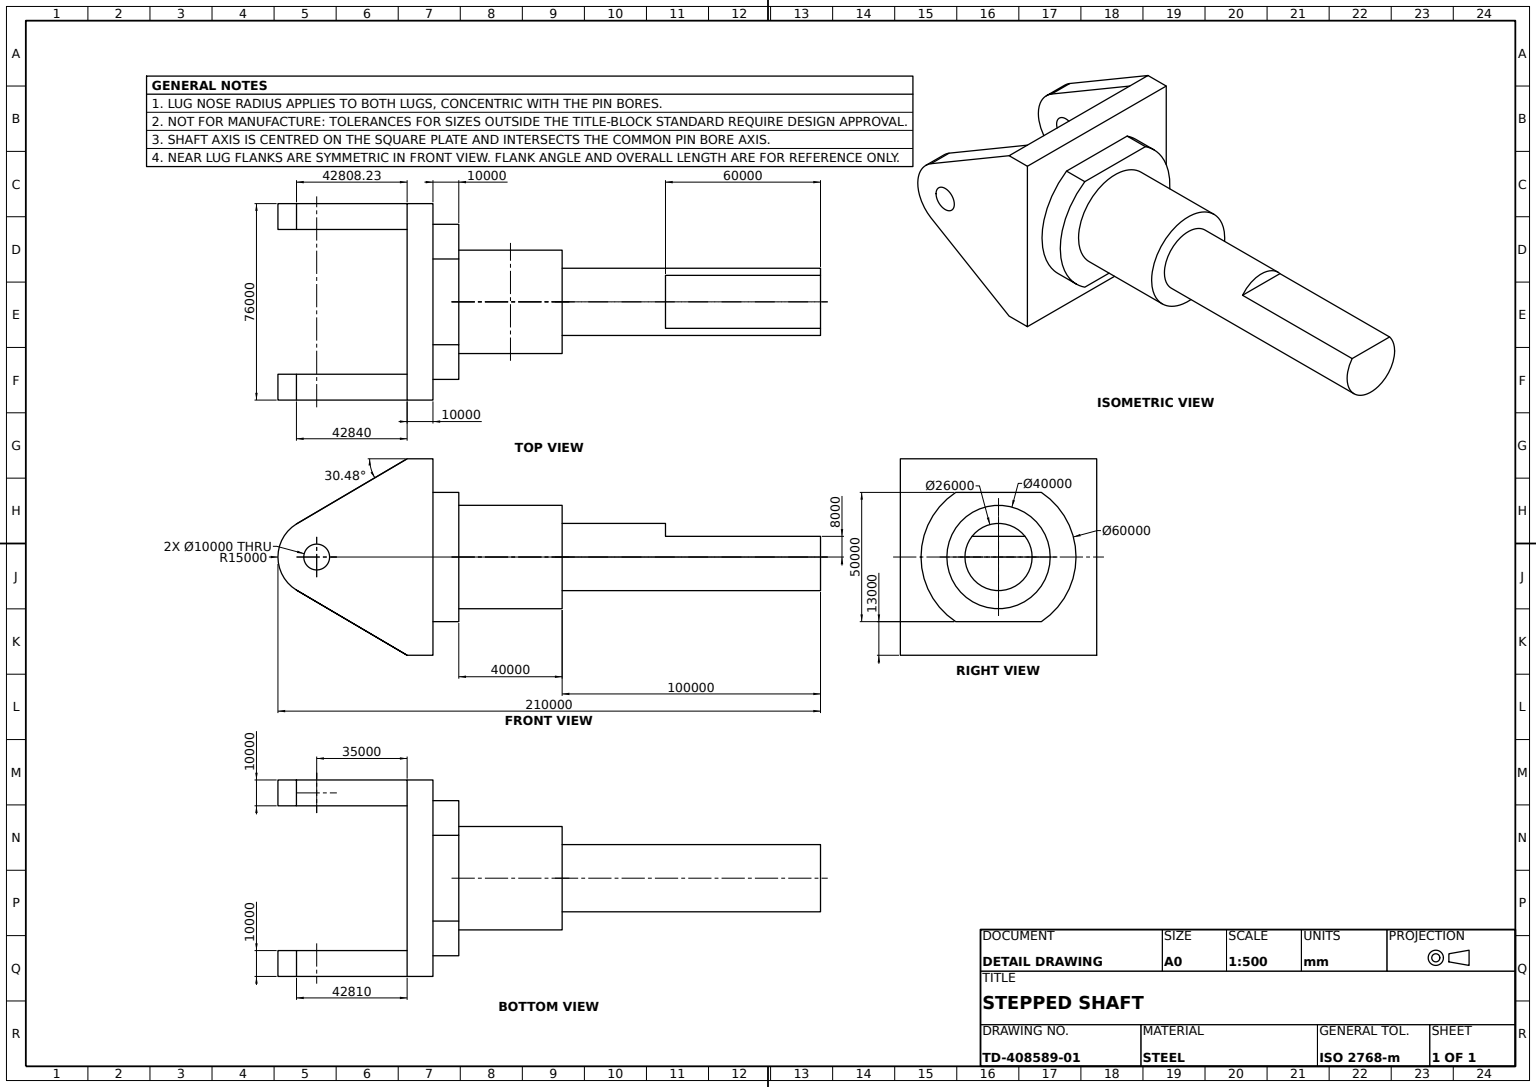
from build123d import *

# Parameters (mm, degrees)
BASE_PLATE_SKETCH_W               = 76000
BASE_PLATE_SKETCH_H               = 76000
BASE_PLATE_DEPTH                  = 10000
CLEVIS_LUG_A_SKETCH_R             = 5000
CLEVIS_LUG_A_DEPTH                = 10000
CLEVIS_START                      = -10000
CLEVIS_LUG_B_SKETCH_R             = 5000
CLEVIS_LUG_B_DEPTH                = 10000
COLLAR_60_SKETCH_R                = 30000
COLLAR_60_DEPTH                   = 10000
HEX_COLLAR_CUT_SKETCH_OUTSIDE_W   = 101655.07
HEX_COLLAR_CUT_SKETCH_OUTSIDE_H   = 101655.07
HEX_COLLAR_CUT_SKETCH_OUTSIDE_W_2 = 70000
HEX_COLLAR_CUT_SKETCH_OUTSIDE_H_2 = 50000
HEX_COLLAR_CUT_DEPTH              = 10000
SHAFT_SHOULDER_40_SKETCH_R        = 20000
SHAFT_SHOULDER_40_DEPTH           = 40000
SHAFT_26_SKETCH_R                 = 13000
SHAFT_26_DEPTH                    = 100000
SHAFT_FLAT_SKETCH_W               = 26683.607246268
SHAFT_FLAT_SKETCH_H               = 10033.036324596
SHAFT_FLAT_CUT_DEPTH              = 60000


with BuildPart() as part:
    # Base Plate Sketch → Base Plate (new body)
    with BuildSketch(Plane.XY):
        Rectangle(BASE_PLATE_SKETCH_W, BASE_PLATE_SKETCH_H)
    extrude(amount=BASE_PLATE_DEPTH)

    # Clevis Lug A Sketch → Clevis Lug A (add)
    with BuildSketch(Plane(origin=(38000, 0, 0), x_dir=(0, 0, -1), z_dir=(1, 0, 0))):
        with BuildLine():
            Line((42405.553807794, 13044.453717955), (0, 38000))
            Line((0, 38000), (0, -38000))
            Line((0, -38000), (42810, -12806.400743378))
            ThreePointArc((42810, -12806.400743378), (49999.999964327, 1.034506538), (42808.233485002, 12807.477887691))
            Line((42808.233485002, 12807.477887691), (42405.553807794, 13044.453717955))
        make_face()
        with Locations((35000, 0)):
            Circle(CLEVIS_LUG_A_SKETCH_R, mode=Mode.SUBTRACT)
    extrude(amount=-CLEVIS_LUG_A_DEPTH)

    # Clevis Lug B Sketch → Clevis Lug B (add)
    with BuildSketch(Plane.ZY.offset(38000).offset(CLEVIS_START)):
        with BuildLine():
            Line((0, 38000), (0, -38000))
            Line((0, -38000), (-42840, -12788.056928244))
            ThreePointArc((-42840, -12788.056928244), (-50000, 0), (-42840, 12788.056928244))
            Line((-42840, 12788.056928244), (0, 38000))
        make_face()
        with Locations(Location((-35000, 0, 0), (0, 0, 180))):
            Circle(CLEVIS_LUG_B_SKETCH_R, mode=Mode.SUBTRACT)
    extrude(amount=CLEVIS_LUG_B_DEPTH)

    # Collar Ø60 Sketch → Collar Ø60 (add)
    with BuildSketch(Plane.XY.offset(10000)):
        Circle(COLLAR_60_SKETCH_R)
    extrude(amount=COLLAR_60_DEPTH)

    # Hex Collar Cut Sketch outside → Hex Collar Cut (cut)
    with BuildSketch(Plane.XY.offset(20000)):
        Rectangle(HEX_COLLAR_CUT_SKETCH_OUTSIDE_W, HEX_COLLAR_CUT_SKETCH_OUTSIDE_H)
        Rectangle(HEX_COLLAR_CUT_SKETCH_OUTSIDE_W_2, HEX_COLLAR_CUT_SKETCH_OUTSIDE_H_2, mode=Mode.SUBTRACT)
    extrude(amount=-HEX_COLLAR_CUT_DEPTH, mode=Mode.SUBTRACT)

    # Shaft Shoulder Ø40 Sketch → Shaft Shoulder Ø40 (add)
    with BuildSketch(Plane.XY.offset(20000)):
        Circle(SHAFT_SHOULDER_40_SKETCH_R)
    extrude(amount=SHAFT_SHOULDER_40_DEPTH)

    # Shaft Ø26 Sketch → Shaft Ø26 (add)
    with BuildSketch(Plane.XY.offset(60000)):
        Circle(SHAFT_26_SKETCH_R)
    extrude(amount=SHAFT_26_DEPTH)

    # Shaft Flat Sketch → Shaft Flat Cut (cut)
    with BuildSketch(Plane.XY.offset(160000)):
        with Locations((0, 13016.518162298)):
            Rectangle(SHAFT_FLAT_SKETCH_W, SHAFT_FLAT_SKETCH_H)
    extrude(amount=-SHAFT_FLAT_CUT_DEPTH, mode=Mode.SUBTRACT)


solid = part.part
